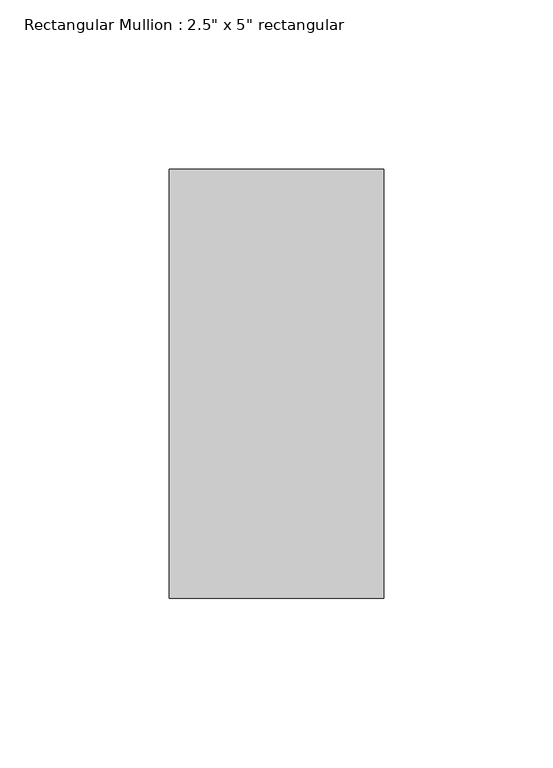
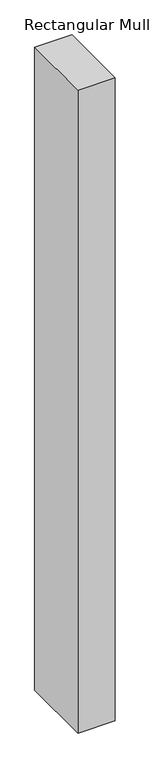
"""IFC4 building model written with IfcOpenShell, lengths in millimetres: member geometry."""

from ifc_helpers import new_model, si_unit, frame, origin, place, context, project, spatial, polyline, outline, extrude, source, transform, mapped, element, save


def member_89a24a7a(model_context):
    return source(origin(), model_context, "Body", "SweptSolid", [
        extrude(outline(polyline([(0.0, 63.5), (0.0, -63.5), (-63.5, -63.5), (-63.5, 63.5), (0.0, 63.5)])), frame((0.0, 0.0, -1155.4992225), z_axis=(0.0, 0.0, 1.0), x_axis=(1.0, 0.0, 0.0)), (0.0, 0.0, 1.0), 1155.4992225),
    ])


if __name__ == "__main__":
    model = new_model("IFC4")
    model_context = context("Model", 3, world=origin())
    ifc_project = project(units=[si_unit("LENGTHUNIT", "METRE", prefix="MILLI")], contexts=[model_context])
    site = spatial("IfcSite", under=ifc_project)
    building = spatial("IfcBuilding", under=site)
    placement = place(None, origin())
    member_shape = member_89a24a7a(model_context)
    element("IfcMember", 1, ObjectType="Rectangular Mullion : 2.5\" x 5\" rectangular", at=placement, inside=building, context=model_context, shape_type="MappedRepresentation", body=[
        mapped(member_shape, transform((0.0, 0.0, 0.0), x_axis=(1.0, 0.0, 0.0), y_axis=(0.0, 1.0, 0.0), z_axis=(0.0, 0.0, 1.0))),
    ])
    save(model, "model.ifc")

# Revit data of these elements
# Type "Rectangular Mullion : 2.5\" x 5\" rectangular"
#   built-in parameter 1007304 = 0.416667 (stored number, unit not read)
#   built-in parameter 1007301 = 0.104167 (stored number, unit not read)
#   built-in parameter 1007300 = 0.104167 (stored number, unit not read)
# Element 1 (IfcMember, "Rectangular Mullion : 2.5\" x 5\" rectangular")
#   Materials on its faces: "Aluminum"
# Materials
#   "Aluminum": class "Metal", colour RGB 247 247 247, transparency 0, Description = "Aluminum 6061", Cost = 0
